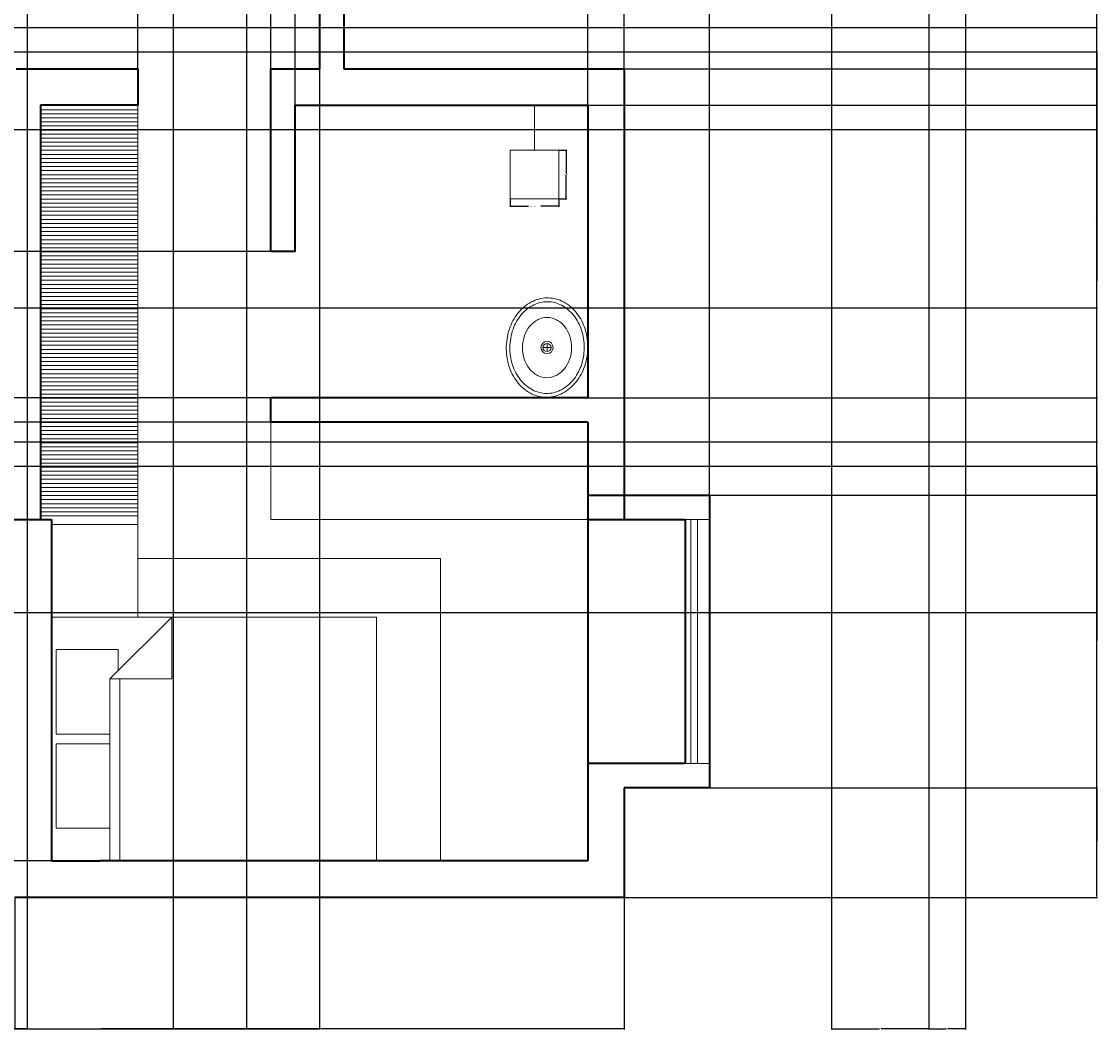
# Model space of a CAD drawing. Units: inches. Extents: x 1159 to 1869, y 2212 to 2738.
# Tile 4 of 5: x 1604 to 1869, y 2212 to 2460. Entities that reach past the tile are written whole.
import ezdxf

# ---------------------------------------------------------------- set-up
doc = ezdxf.new("R2010")
doc.units = ezdxf.units.IN
for name, color, linetype, lineweight in [('A-ANNO-DIMS', 2, 'Continuous', 18), ('A-FLOR', 9, 'Continuous', 13), ('A-FLOR-CASE', 30, 'Continuous', 18), ('A-FLOR-FIXT', 9, 'Continuous', 18), ('A-FLOR-PATT', 252, 'Continuous', 13), ('A-FURN', 8, 'Continuous', 18), ('A-GLAZ', 4, 'Continuous', 18), ('A-WALL', 7, 'Continuous', 35)]:
    doc.layers.add(name, color=color, linetype=linetype, lineweight=lineweight)
doc.styles.get("Standard").update_dxf_attribs({"font": 'arial.ttf'})
doc.dimstyles.get("Standard").update_dxf_attribs({"dimtxt": 0.18, "dimasz": 0.18, "dimexe": 0.18, "dimexo": 0.0625, "dimgap": 0.09, "dimtad": 0, "dimtih": 1, "dimtoh": 1, "dimdec": 4, "dimzin": 0, "dimdsep": 46, "dimtxsty": 'Standard', "dimcen": 0.09, "dimadec": 0, "dimazin": 0, "dimtfac": 1, "dimtdec": 4, "dimtofl": 0, "dimtmove": 0, "dimatfit": 3, "dimfxl": 1, "dimtolj": 1, "dimtzin": 0, "dimarcsym": 0})

# ---------------------------------------------------------------- blocks, each defined once
blk = doc.blocks.new('Bed - Queen')
for p, q in [((0, -80.00003), (0, 0)), ((0, 0), (59.99999, 0)), ((59.99999, 0), (59.99999, -80.00003)), ((7.99999, -1.2), (28.79998, -1.2)), ((7.99999, -14.4), (7.99999, -1.2)), ((28.79998, -1.2), (28.79998, -14.4)), ((31.19999, -1.2), (51.99999, -1.2)), ((31.19999, -14.4), (31.19999, -1.2)), ((51.99999, -1.2), (51.99999, -16.4)), ((0, -14.4), (44.8, -14.4)), ((59.99999, -29.6), (44.8, -14.4)), ((44.8, -14.4), (44.8, -29.6)), ((44.8, -16.8), (0, -16.8)), ((51.99999, -16.4), (46.79936, -16.4)), ((44.8, -29.6), (59.99999, -29.6)), ((59.99999, -80.00003), (0, -80.00003))]:
    blk.add_line(p, q)
blk = doc.blocks.new('Sink - Oval top')
for p, q in [((-1, 0), (1, 0)), ((0, 1), (0, -1))]:
    blk.add_line(p, q)
for points in [[(-12.23, 0.39, 0.117634), (-11.46, -3.36, 0.104469), (-8.88, -6.8, 0.090016), (-5.08, -9.07, 0.08192), (-0.32, -10.02, 0.08192), (4.49, -9.38, 0.090016), (8.42, -7.36, 0.104469), (11.22, -4.09, 0.117634), (12.23, -0.39, 0.117634), (11.46, 3.36, 0.104469), (8.88, 6.8, 0.090016), (5.08, 9.07, 0.08192), (0.32, 10.02, 0.08192), (-4.49, 9.38, 0.090016), (-8.42, 7.36, 0.104469), (-11.22, 4.09, 0.117634)], [(-11.29, 0.16, 0.118622), (-10.52, -3.25, 0.104678), (-8.07, -6.36, 0.089562), (-4.54, -8.37, 0.081185), (-0.13, -9.15, 0.081185), (4.3, -8.49, 0.089562), (7.89, -6.58, 0.104678), (10.42, -3.55, 0.118622), (11.29, -0.16, 0.118622), (10.52, 3.25, 0.104678), (8.07, 6.36, 0.089562), (4.54, 8.37, 0.081185), (0.13, 9.15, 0.081185), (-4.3, 8.49, 0.089562), (-7.89, 6.58, 0.104678), (-10.42, 3.55, 0.118622)], [(-7.42, 0.08, 0.118283), (-6.91, -2.17, 0.104607), (-5.29, -4.21, 0.089718), (-2.97, -5.53, 0.081436), (-0.07, -6.04, 0.081436), (2.84, -5.59, 0.089718), (5.2, -4.33, 0.104607), (6.86, -2.32, 0.118283), (7.42, -0.08, 0.118283), (6.91, 2.17, 0.104607), (5.29, 4.21, 0.089718), (2.97, 5.53, 0.081436), (0.07, 6.04, 0.081436), (-2.84, 5.59, 0.089718), (-5.2, 4.33, 0.104607), (-6.86, 2.32, 0.118283)]]:
    blk.add_lwpolyline(points, format="xyb", close=True)
for radius in [1.5, 1]:
    blk.add_circle((0, 0), radius)
blk = doc.blocks.new('SHOWER-HEAD-SQUARE-12IN')
for p, q in [((6, 12), (0, 12)), ((0, 12), (0, 0)), ((12, 12), (6, 12)), ((12, 0), (12, 12)), ((0, 0), (12, 0))]:
    blk.add_line(p, q)
blk = doc.blocks.new('*D12')
at = {"layer": 'A-ANNO-DIMS', "color": 0, "lineweight": -2, "transparency": 16777216}
for p, q in [((1724.31, 2415.97), (1724.31, 2414.05)), ((1736.31, 2415.97), (1736.31, 2414.05)), ((1724.49, 2414.23), (1728.8, 2414.23)), ((1736.13, 2414.23), (1731.82, 2414.23))]:
    blk.add_line(p, q, dxfattribs=at)
at = {"layer": 'A-ANNO-DIMS', "color": 0, "transparency": 16777216}
for points in [[(1724.49, 2414.26), (1724.49, 2414.2), (1724.31, 2414.23)], [(1736.13, 2414.26), (1736.13, 2414.2), (1736.31, 2414.23)]]:
    blk.add_solid(points, dxfattribs=at)
at = {"layer": 'Defpoints', "color": 0, "transparency": 16777216}
for p in [(1724.31, 2416.03), (1736.31, 2416.03), (1736.31, 2414.23)]:
    blk.add_point(p, dxfattribs=at)
at = {"layer": 'A-ANNO-DIMS', "color": 0, "transparency": 16777216, "insert": (1730.31, 2414.23), "char_height": 0.18, "attachment_point": 5}
blk.add_mtext('\\A1;SHOWER HEAD 12 TYP.', dxfattribs=at)
blk = doc.blocks.new('*D13')
at = {"layer": 'A-ANNO-DIMS', "color": 0, "lineweight": -2, "transparency": 16777216}
for p, q in [((1736.37, 2428.03), (1738.29, 2428.03)), ((1738.11, 2427.85), (1738.11, 2422.21)), ((1738.11, 2416.21), (1738.11, 2421.85)), ((1736.37, 2416.03), (1738.29, 2416.03))]:
    blk.add_line(p, q, dxfattribs=at)
at = {"layer": 'A-ANNO-DIMS', "color": 0, "transparency": 16777216}
for points in [[(1738.08, 2427.85), (1738.14, 2427.85), (1738.11, 2428.03)], [(1738.08, 2416.21), (1738.14, 2416.21), (1738.11, 2416.03)]]:
    blk.add_solid(points, dxfattribs=at)
at = {"layer": 'Defpoints', "color": 0, "transparency": 16777216}
for p in [(1736.31, 2428.03), (1738.11, 2428.03), (1736.31, 2416.03)]:
    blk.add_point(p, dxfattribs=at)
at = {"layer": 'A-ANNO-DIMS', "color": 0, "transparency": 16777216, "insert": (1738.11, 2422.03), "char_height": 0.18, "attachment_point": 5}
blk.add_mtext('\\A1;12 TYP.', dxfattribs=at)
blk = doc.blocks.new('*D21')
at = {"layer": 'A-ANNO-DIMS', "color": 0, "lineweight": -2, "transparency": 16777216}
for p, q in [((1836.46, 2705.63), (1868.92, 2705.63)), ((1868.74, 2705.45), (1868.74, 2475.03)), ((1868.74, 2244.26), (1868.74, 2474.67)), ((1752.46, 2244.08), (1868.92, 2244.08))]:
    blk.add_line(p, q, dxfattribs=at)
at = {"layer": 'A-ANNO-DIMS', "color": 0, "transparency": 16777216}
for points in [[(1868.71, 2705.45), (1868.77, 2705.45), (1868.74, 2705.63)], [(1868.71, 2244.26), (1868.77, 2244.26), (1868.74, 2244.08)]]:
    blk.add_solid(points, dxfattribs=at)
at = {"layer": 'Defpoints', "color": 0, "transparency": 16777216}
for p in [(1836.4, 2705.63), (1868.74, 2705.63), (1752.4, 2244.08)]:
    blk.add_point(p, dxfattribs=at)
at = {"layer": 'A-ANNO-DIMS', "color": 0, "transparency": 16777216, "insert": (1868.74, 2474.85), "char_height": 0.18, "attachment_point": 5}
blk.add_mtext('\\A1;461.55', dxfattribs=at)
blk = doc.blocks.new('*D28')
at = {"layer": 'A-ANNO-DIMS', "color": 0, "lineweight": -2, "transparency": 16777216}
for p, q in [((1602.4, 2244.01), (1602.4, 2211.56)), ((1752.4, 2244.01), (1752.4, 2211.56)), ((1602.58, 2211.74), (1677.12, 2211.74)), ((1752.22, 2211.74), (1677.68, 2211.74))]:
    blk.add_line(p, q, dxfattribs=at)
at = {"layer": 'A-ANNO-DIMS', "color": 0, "transparency": 16777216}
for points in [[(1602.58, 2211.77), (1602.58, 2211.71), (1602.4, 2211.74)], [(1752.22, 2211.77), (1752.22, 2211.71), (1752.4, 2211.74)]]:
    blk.add_solid(points, dxfattribs=at)
at = {"layer": 'Defpoints', "color": 0, "transparency": 16777216}
for p in [(1602.4, 2244.08), (1752.4, 2244.08), (1752.4, 2211.74)]:
    blk.add_point(p, dxfattribs=at)
at = {"layer": 'A-ANNO-DIMS', "color": 0, "transparency": 16777216, "insert": (1677.4, 2211.74), "char_height": 0.18, "attachment_point": 5}
blk.add_mtext('\\A1;150', dxfattribs=at)
blk = doc.blocks.new('*D31')
at = {"layer": 'A-ANNO-DIMS', "color": 0, "lineweight": -2, "transparency": 16777216}
for p, q in [((1698.46, 2519.63), (1868.92, 2519.63)), ((1868.74, 2519.45), (1868.74, 2484.03)), ((1868.74, 2448.26), (1868.74, 2483.67)), ((1683.46, 2448.08), (1868.92, 2448.08))]:
    blk.add_line(p, q, dxfattribs=at)
at = {"layer": 'A-ANNO-DIMS', "color": 0, "transparency": 16777216}
for points in [[(1868.71, 2519.45), (1868.77, 2519.45), (1868.74, 2519.63)], [(1868.71, 2448.26), (1868.77, 2448.26), (1868.74, 2448.08)]]:
    blk.add_solid(points, dxfattribs=at)
at = {"layer": 'Defpoints', "color": 0, "transparency": 16777216}
for p in [(1698.4, 2519.63), (1683.4, 2448.08), (1868.74, 2448.08)]:
    blk.add_point(p, dxfattribs=at)
at = {"layer": 'A-ANNO-DIMS', "color": 0, "transparency": 16777216, "insert": (1868.74, 2483.85), "char_height": 0.18, "attachment_point": 5}
blk.add_mtext('\\A1;71.55', dxfattribs=at)
blk = doc.blocks.new('*D33')
at = {"layer": 'A-ANNO-DIMS', "color": 0, "lineweight": -2, "transparency": 16777216}
for p, q in [((1773.46, 2271.08), (1868.92, 2271.08)), ((1868.74, 2270.9), (1868.74, 2257.76)), ((1868.74, 2244.26), (1868.74, 2257.4)), ((1752.46, 2244.08), (1868.92, 2244.08))]:
    blk.add_line(p, q, dxfattribs=at)
at = {"layer": 'A-ANNO-DIMS', "color": 0, "transparency": 16777216}
for points in [[(1868.71, 2270.9), (1868.77, 2270.9), (1868.74, 2271.08)], [(1868.71, 2244.26), (1868.77, 2244.26), (1868.74, 2244.08)]]:
    blk.add_solid(points, dxfattribs=at)
at = {"layer": 'Defpoints', "color": 0, "transparency": 16777216}
for p in [(1773.4, 2271.08), (1868.74, 2271.08), (1752.4, 2244.08)]:
    blk.add_point(p, dxfattribs=at)
at = {"layer": 'A-ANNO-DIMS', "color": 0, "transparency": 16777216, "insert": (1868.74, 2257.58), "char_height": 0.18, "attachment_point": 5}
blk.add_mtext('\\A1;27', dxfattribs=at)
blk = doc.blocks.new('*D34')
at = {"layer": 'A-ANNO-DIMS', "color": 0, "lineweight": -2, "transparency": 16777216}
for p, q in [((1773.46, 2343.08), (1868.92, 2343.08)), ((1868.74, 2342.9), (1868.74, 2307.26)), ((1868.74, 2271.26), (1868.74, 2306.9)), ((1773.46, 2271.08), (1868.92, 2271.08))]:
    blk.add_line(p, q, dxfattribs=at)
at = {"layer": 'A-ANNO-DIMS', "color": 0, "transparency": 16777216}
for points in [[(1868.71, 2342.9), (1868.77, 2342.9), (1868.74, 2343.08)], [(1868.71, 2271.26), (1868.77, 2271.26), (1868.74, 2271.08)]]:
    blk.add_solid(points, dxfattribs=at)
at = {"layer": 'Defpoints', "color": 0, "transparency": 16777216}
for p in [(1773.4, 2343.08), (1868.74, 2343.08), (1773.4, 2271.08)]:
    blk.add_point(p, dxfattribs=at)
at = {"layer": 'A-ANNO-DIMS', "color": 0, "transparency": 16777216, "insert": (1868.74, 2307.08), "char_height": 0.18, "attachment_point": 5}
blk.add_mtext('\\A1;72', dxfattribs=at)
blk = doc.blocks.new('*D35')
at = {"layer": 'A-ANNO-DIMS', "color": 0, "lineweight": -2, "transparency": 16777216}
for p, q in [((1752.46, 2448.08), (1868.92, 2448.08)), ((1868.74, 2447.9), (1868.74, 2395.76)), ((1868.74, 2343.26), (1868.74, 2395.39)), ((1773.46, 2343.08), (1868.92, 2343.08))]:
    blk.add_line(p, q, dxfattribs=at)
at = {"layer": 'A-ANNO-DIMS', "color": 0, "transparency": 16777216}
for points in [[(1868.71, 2447.9), (1868.77, 2447.9), (1868.74, 2448.08)], [(1868.71, 2343.26), (1868.77, 2343.26), (1868.74, 2343.08)]]:
    blk.add_solid(points, dxfattribs=at)
at = {"layer": 'Defpoints', "color": 0, "transparency": 16777216}
for p in [(1752.4, 2448.08), (1868.74, 2448.08), (1773.4, 2343.08)]:
    blk.add_point(p, dxfattribs=at)
at = {"layer": 'A-ANNO-DIMS', "color": 0, "transparency": 16777216, "insert": (1868.74, 2395.58), "char_height": 0.18, "attachment_point": 5}
blk.add_mtext('\\A1;105', dxfattribs=at)
blk = doc.blocks.new('*D36')
at = {"layer": 'A-ANNO-DIMS', "color": 0, "lineweight": -2, "transparency": 16777216}
for p, q in [((1752.4, 2337.14), (1752.4, 2738.15)), ((1752.58, 2737.97), (1762.7, 2737.97)), ((1773.22, 2737.97), (1763.1, 2737.97)), ((1773.4, 2343.14), (1773.4, 2738.15))]:
    blk.add_line(p, q, dxfattribs=at)
at = {"layer": 'A-ANNO-DIMS', "color": 0, "transparency": 16777216}
for points in [[(1752.58, 2738), (1752.58, 2737.94), (1752.4, 2737.97)], [(1773.22, 2738), (1773.22, 2737.94), (1773.4, 2737.97)]]:
    blk.add_solid(points, dxfattribs=at)
at = {"layer": 'Defpoints', "color": 0, "transparency": 16777216}
for p in [(1773.4, 2737.97), (1773.4, 2343.08), (1752.4, 2337.08)]:
    blk.add_point(p, dxfattribs=at)
at = {"layer": 'A-ANNO-DIMS', "color": 0, "transparency": 16777216, "insert": (1762.9, 2737.97), "char_height": 0.18, "attachment_point": 5}
blk.add_mtext('\\A1;21', dxfattribs=at)
blk = doc.blocks.new('*D39')
at = {"layer": 'A-ANNO-DIMS', "color": 0, "lineweight": -2, "transparency": 16777216}
for p, q in [((1605.4, 2696.57), (1605.4, 2211.56)), ((1677.4, 2696.57), (1677.4, 2211.56)), ((1605.58, 2211.74), (1641.18, 2211.74)), ((1677.22, 2211.74), (1641.62, 2211.74))]:
    blk.add_line(p, q, dxfattribs=at)
at = {"layer": 'A-ANNO-DIMS', "color": 0, "transparency": 16777216}
for points in [[(1605.58, 2211.77), (1605.58, 2211.71), (1605.4, 2211.74)], [(1677.22, 2211.77), (1677.22, 2211.71), (1677.4, 2211.74)]]:
    blk.add_solid(points, dxfattribs=at)
at = {"layer": 'Defpoints', "color": 0, "transparency": 16777216}
for p in [(1605.4, 2696.63), (1677.4, 2696.63), (1677.4, 2211.74)]:
    blk.add_point(p, dxfattribs=at)
at = {"layer": 'A-ANNO-DIMS', "color": 0, "transparency": 16777216, "insert": (1641.4, 2211.74), "char_height": 0.18, "attachment_point": 5}
blk.add_mtext('\\A1;72', dxfattribs=at)
blk = doc.blocks.new('*D42')
at = {"layer": 'A-ANNO-DIMS', "color": 0, "lineweight": -2, "transparency": 16777216}
for p, q in [((1200.46, 2452.21), (1868.92, 2452.21)), ((1868.74, 2452.03), (1868.74, 2404.39)), ((1868.74, 2356.39), (1868.74, 2404.02)), ((1200.46, 2356.21), (1868.92, 2356.21))]:
    blk.add_line(p, q, dxfattribs=at)
at = {"layer": 'A-ANNO-DIMS', "color": 0, "transparency": 16777216}
for points in [[(1868.71, 2452.03), (1868.77, 2452.03), (1868.74, 2452.21)], [(1868.71, 2356.39), (1868.77, 2356.39), (1868.74, 2356.21)]]:
    blk.add_solid(points, dxfattribs=at)
at = {"layer": 'Defpoints', "color": 0, "transparency": 16777216}
for p in [(1200.4, 2452.21), (1868.74, 2452.21), (1200.4, 2356.21)]:
    blk.add_point(p, dxfattribs=at)
at = {"layer": 'A-ANNO-DIMS', "color": 0, "transparency": 16777216, "insert": (1868.74, 2404.21), "char_height": 0.18, "attachment_point": 5}
blk.add_mtext('\\A1;96', dxfattribs=at)
blk = doc.blocks.new('*D43')
at = {"layer": 'A-ANNO-DIMS', "color": 0, "lineweight": -2, "transparency": 16777216}
for p, q in [((1671.4, 2439.14), (1671.4, 2738.15)), ((1671.58, 2737.97), (1707.18, 2737.97)), ((1743.22, 2737.97), (1707.62, 2737.97)), ((1743.4, 2439.14), (1743.4, 2738.15))]:
    blk.add_line(p, q, dxfattribs=at)
at = {"layer": 'A-ANNO-DIMS', "color": 0, "transparency": 16777216}
for points in [[(1671.58, 2738), (1671.58, 2737.94), (1671.4, 2737.97)], [(1743.22, 2738), (1743.22, 2737.94), (1743.4, 2737.97)]]:
    blk.add_solid(points, dxfattribs=at)
at = {"layer": 'Defpoints', "color": 0, "transparency": 16777216}
for p in [(1743.4, 2737.97), (1671.4, 2439.08), (1743.4, 2439.08)]:
    blk.add_point(p, dxfattribs=at)
at = {"layer": 'A-ANNO-DIMS', "color": 0, "transparency": 16777216, "insert": (1707.4, 2737.97), "char_height": 0.18, "attachment_point": 5}
blk.add_mtext('\\A1;72', dxfattribs=at)
blk = doc.blocks.new('*D44')
at = {"layer": 'A-ANNO-DIMS', "color": 0, "lineweight": -2, "transparency": 16777216}
for p, q in [((1671.46, 2439.08), (1868.92, 2439.08)), ((1868.74, 2438.9), (1868.74, 2403.26)), ((1868.74, 2367.26), (1868.74, 2402.9)), ((1671.46, 2367.08), (1868.92, 2367.08))]:
    blk.add_line(p, q, dxfattribs=at)
at = {"layer": 'A-ANNO-DIMS', "color": 0, "transparency": 16777216}
for points in [[(1868.71, 2438.9), (1868.77, 2438.9), (1868.74, 2439.08)], [(1868.71, 2367.26), (1868.77, 2367.26), (1868.74, 2367.08)]]:
    blk.add_solid(points, dxfattribs=at)
at = {"layer": 'Defpoints', "color": 0, "transparency": 16777216}
for p in [(1671.4, 2439.08), (1868.74, 2439.08), (1671.4, 2367.08)]:
    blk.add_point(p, dxfattribs=at)
at = {"layer": 'A-ANNO-DIMS', "color": 0, "transparency": 16777216, "insert": (1868.74, 2403.08), "char_height": 0.18, "attachment_point": 5}
blk.add_mtext('\\A1;72', dxfattribs=at)
blk = doc.blocks.new('*D53')
at = {"layer": 'A-ANNO-DIMS', "color": 0, "lineweight": -2, "transparency": 16777216}
for p, q in [((1425.46, 2504.63), (1868.92, 2504.63)), ((1868.74, 2504.45), (1868.74, 2481.6)), ((1868.74, 2458.39), (1868.74, 2481.24)), ((1428.81, 2458.21), (1868.92, 2458.21))]:
    blk.add_line(p, q, dxfattribs=at)
at = {"layer": 'A-ANNO-DIMS', "color": 0, "transparency": 16777216}
for points in [[(1868.71, 2504.45), (1868.77, 2504.45), (1868.74, 2504.63)], [(1868.71, 2458.39), (1868.77, 2458.39), (1868.74, 2458.21)]]:
    blk.add_solid(points, dxfattribs=at)
at = {"layer": 'Defpoints', "color": 0, "transparency": 16777216}
for p in [(1425.4, 2504.63), (1868.74, 2504.63), (1428.74, 2458.21)]:
    blk.add_point(p, dxfattribs=at)
at = {"layer": 'A-ANNO-DIMS', "color": 0, "transparency": 16777216, "insert": (1868.74, 2481.42), "char_height": 0.18, "attachment_point": 5}
blk.add_mtext('\\A1;46.42', dxfattribs=at)
blk = doc.blocks.new('*D58')
at = {"layer": 'A-ANNO-DIMS', "color": 0, "lineweight": -2, "transparency": 16777216}
for p, q in [((1538.03, 2433.09), (1868.92, 2433.09)), ((1868.74, 2432.91), (1868.74, 2411.32)), ((1868.74, 2389.36), (1868.74, 2410.95)), ((1538.03, 2389.18), (1868.92, 2389.18))]:
    blk.add_line(p, q, dxfattribs=at)
at = {"layer": 'A-ANNO-DIMS', "color": 0, "transparency": 16777216}
for points in [[(1868.71, 2432.91), (1868.77, 2432.91), (1868.74, 2433.09)], [(1868.71, 2389.36), (1868.77, 2389.36), (1868.74, 2389.18)]]:
    blk.add_solid(points, dxfattribs=at)
at = {"layer": 'Defpoints', "color": 0, "transparency": 16777216}
for p in [(1537.97, 2433.09), (1868.74, 2433.09), (1537.97, 2389.18)]:
    blk.add_point(p, dxfattribs=at)
at = {"layer": 'A-ANNO-DIMS', "color": 0, "transparency": 16777216, "insert": (1868.74, 2411.14), "char_height": 0.18, "attachment_point": 5}
blk.add_mtext('\\A1;43.92', dxfattribs=at)
blk = doc.blocks.new('*D60')
at = {"layer": 'A-ANNO-DIMS', "color": 0, "lineweight": -2, "transparency": 16777216}
for p, q in [((1659.4, 2552.57), (1659.4, 2211.56)), ((1605.4, 2549.57), (1605.4, 2211.56)), ((1605.58, 2211.74), (1632.18, 2211.74)), ((1659.22, 2211.74), (1632.62, 2211.74))]:
    blk.add_line(p, q, dxfattribs=at)
at = {"layer": 'A-ANNO-DIMS', "color": 0, "transparency": 16777216}
for points in [[(1605.58, 2211.77), (1605.58, 2211.71), (1605.4, 2211.74)], [(1659.22, 2211.77), (1659.22, 2211.71), (1659.4, 2211.74)]]:
    blk.add_solid(points, dxfattribs=at)
at = {"layer": 'Defpoints', "color": 0, "transparency": 16777216}
for p in [(1659.4, 2552.63), (1605.4, 2549.63), (1605.4, 2211.74)]:
    blk.add_point(p, dxfattribs=at)
at = {"layer": 'A-ANNO-DIMS', "color": 0, "transparency": 16777216, "insert": (1632.4, 2211.74), "char_height": 0.18, "attachment_point": 5}
blk.add_mtext('\\A1;54', dxfattribs=at)
blk = doc.blocks.new('*D61')
at = {"layer": 'A-ANNO-DIMS', "color": 0, "lineweight": -2, "transparency": 16777216}
for p, q in [((1632.68, 2448.14), (1632.68, 2738.15)), ((1632.86, 2737.97), (1648.65, 2737.97)), ((1665.22, 2737.97), (1649.43, 2737.97)), ((1665.4, 2448.14), (1665.4, 2738.15))]:
    blk.add_line(p, q, dxfattribs=at)
at = {"layer": 'A-ANNO-DIMS', "color": 0, "transparency": 16777216}
for points in [[(1632.86, 2738), (1632.86, 2737.94), (1632.68, 2737.97)], [(1665.22, 2738), (1665.22, 2737.94), (1665.4, 2737.97)]]:
    blk.add_solid(points, dxfattribs=at)
at = {"layer": 'Defpoints', "color": 0, "transparency": 16777216}
for p in [(1665.4, 2737.97), (1632.68, 2448.08), (1665.4, 2448.08)]:
    blk.add_point(p, dxfattribs=at)
at = {"layer": 'A-ANNO-DIMS', "color": 0, "transparency": 16777216, "insert": (1649.04, 2737.97), "char_height": 0.18, "attachment_point": 5}
blk.add_mtext('\\A1;32.72', dxfattribs=at)
blk = doc.blocks.new('*D65')
at = {"layer": 'A-ANNO-DIMS', "color": 0, "lineweight": -2, "transparency": 16777216}
for p, q in [((1542.76, 2504.57), (1542.76, 2211.56)), ((1605.4, 2504.57), (1605.4, 2211.56)), ((1542.94, 2211.74), (1573.69, 2211.74)), ((1605.22, 2211.74), (1574.48, 2211.74))]:
    blk.add_line(p, q, dxfattribs=at)
at = {"layer": 'A-ANNO-DIMS', "color": 0, "transparency": 16777216}
for points in [[(1542.94, 2211.77), (1542.94, 2211.71), (1542.76, 2211.74)], [(1605.22, 2211.77), (1605.22, 2211.71), (1605.4, 2211.74)]]:
    blk.add_solid(points, dxfattribs=at)
at = {"layer": 'Defpoints', "color": 0, "transparency": 16777216}
for p in [(1542.76, 2504.63), (1605.4, 2504.63), (1605.4, 2211.74)]:
    blk.add_point(p, dxfattribs=at)
at = {"layer": 'A-ANNO-DIMS', "color": 0, "transparency": 16777216, "insert": (1574.08, 2211.74), "char_height": 0.18, "attachment_point": 5}
blk.add_mtext('\\A1;62.64', dxfattribs=at)
blk = doc.blocks.new('*D66')
at = {"layer": 'A-ANNO-DIMS', "color": 0, "lineweight": -2, "transparency": 16777216}
for p, q in [((1605.4, 2696.57), (1605.4, 2211.56)), ((1641.4, 2600.57), (1641.4, 2211.56)), ((1605.58, 2211.74), (1623.18, 2211.74)), ((1641.22, 2211.74), (1623.62, 2211.74))]:
    blk.add_line(p, q, dxfattribs=at)
at = {"layer": 'A-ANNO-DIMS', "color": 0, "transparency": 16777216}
for points in [[(1605.58, 2211.77), (1605.58, 2211.71), (1605.4, 2211.74)], [(1641.22, 2211.77), (1641.22, 2211.71), (1641.4, 2211.74)]]:
    blk.add_solid(points, dxfattribs=at)
at = {"layer": 'Defpoints', "color": 0, "transparency": 16777216}
for p in [(1605.4, 2696.63), (1641.4, 2600.63), (1605.4, 2211.74)]:
    blk.add_point(p, dxfattribs=at)
at = {"layer": 'A-ANNO-DIMS', "color": 0, "transparency": 16777216, "insert": (1623.4, 2211.74), "char_height": 0.18, "attachment_point": 5}
blk.add_mtext('\\A1;36', dxfattribs=at)
blk = doc.blocks.new('*D67')
at = {"layer": 'A-ANNO-DIMS', "color": 0, "lineweight": -2, "transparency": 16777216}
for p, q in [((1665.34, 2403.08), (1158.88, 2403.08)), ((1159.06, 2402.9), (1159.06, 2385.26)), ((1159.06, 2367.26), (1159.06, 2384.89)), ((1665.34, 2367.08), (1158.88, 2367.08))]:
    blk.add_line(p, q, dxfattribs=at)
at = {"layer": 'A-ANNO-DIMS', "color": 0, "transparency": 16777216}
for points in [[(1159.03, 2402.9), (1159.09, 2402.9), (1159.06, 2403.08)], [(1159.03, 2367.26), (1159.09, 2367.26), (1159.06, 2367.08)]]:
    blk.add_solid(points, dxfattribs=at)
at = {"layer": 'Defpoints', "color": 0, "transparency": 16777216}
for p in [(1159.06, 2403.08), (1665.4, 2403.08), (1665.4, 2367.08)]:
    blk.add_point(p, dxfattribs=at)
at = {"layer": 'A-ANNO-DIMS', "color": 0, "transparency": 16777216, "insert": (1159.06, 2385.08), "char_height": 0.18, "attachment_point": 5}
blk.add_mtext('\\A1;36', dxfattribs=at)
blk = doc.blocks.new('*D68')
at = {"layer": 'A-ANNO-DIMS', "color": 0, "lineweight": -2, "transparency": 16777216}
for p, q in [((1803.4, 2552.57), (1803.4, 2211.56)), ((1827.4, 2552.57), (1827.4, 2211.56)), ((1803.58, 2211.74), (1815.18, 2211.74)), ((1827.22, 2211.74), (1815.62, 2211.74))]:
    blk.add_line(p, q, dxfattribs=at)
at = {"layer": 'A-ANNO-DIMS', "color": 0, "transparency": 16777216}
for points in [[(1803.58, 2211.77), (1803.58, 2211.71), (1803.4, 2211.74)], [(1827.22, 2211.77), (1827.22, 2211.71), (1827.4, 2211.74)]]:
    blk.add_solid(points, dxfattribs=at)
at = {"layer": 'Defpoints', "color": 0, "transparency": 16777216}
for p in [(1803.4, 2552.63), (1827.4, 2552.63), (1827.4, 2211.74)]:
    blk.add_point(p, dxfattribs=at)
at = {"layer": 'A-ANNO-DIMS', "color": 0, "transparency": 16777216, "insert": (1815.4, 2211.74), "char_height": 0.18, "attachment_point": 5}
blk.add_mtext('\\A1;24', dxfattribs=at)
blk = doc.blocks.new('*D70')
at = {"layer": 'A-ANNO-DIMS', "color": 0, "lineweight": -2, "transparency": 16777216}
for p, q in [((1827.4, 2528.57), (1827.4, 2211.56)), ((1836.4, 2519.57), (1836.4, 2211.56)), ((1827.58, 2211.74), (1831.75, 2211.74)), ((1836.22, 2211.74), (1832.05, 2211.74))]:
    blk.add_line(p, q, dxfattribs=at)
at = {"layer": 'A-ANNO-DIMS', "color": 0, "transparency": 16777216}
for points in [[(1827.58, 2211.77), (1827.58, 2211.71), (1827.4, 2211.74)], [(1836.22, 2211.77), (1836.22, 2211.71), (1836.4, 2211.74)]]:
    blk.add_solid(points, dxfattribs=at)
at = {"layer": 'Defpoints', "color": 0, "transparency": 16777216}
for p in [(1827.4, 2528.63), (1836.4, 2519.63), (1836.4, 2211.74)]:
    blk.add_point(p, dxfattribs=at)
at = {"layer": 'A-ANNO-DIMS', "color": 0, "transparency": 16777216, "insert": (1831.9, 2211.74), "char_height": 0.18, "attachment_point": 5}
blk.add_mtext('\\A1;9', dxfattribs=at)
blk = doc.blocks.new('*D71')
at = {"layer": 'A-ANNO-DIMS', "color": 0, "lineweight": -2, "transparency": 16777216}
for p, q in [((1677.4, 2448.14), (1677.4, 2738.15)), ((1677.58, 2737.97), (1680.25, 2737.97)), ((1683.22, 2737.97), (1680.55, 2737.97)), ((1683.4, 2448.14), (1683.4, 2738.15))]:
    blk.add_line(p, q, dxfattribs=at)
at = {"layer": 'A-ANNO-DIMS', "color": 0, "transparency": 16777216}
for points in [[(1677.58, 2738), (1677.58, 2737.94), (1677.4, 2737.97)], [(1683.22, 2738), (1683.22, 2737.94), (1683.4, 2737.97)]]:
    blk.add_solid(points, dxfattribs=at)
at = {"layer": 'Defpoints', "color": 0, "transparency": 16777216}
for p in [(1683.4, 2737.97), (1677.4, 2448.08), (1683.4, 2448.08)]:
    blk.add_point(p, dxfattribs=at)
at = {"layer": 'A-ANNO-DIMS', "color": 0, "transparency": 16777216, "insert": (1680.4, 2737.97), "char_height": 0.18, "attachment_point": 5}
blk.add_mtext('\\A1;6', dxfattribs=at)
blk = doc.blocks.new('*D74')
at = {"layer": 'A-ANNO-DIMS', "color": 0, "lineweight": -2, "transparency": 16777216}
for p, q in [((1743.34, 2361.08), (1158.88, 2361.08)), ((1159.06, 2360.9), (1159.06, 2307.26)), ((1159.06, 2253.26), (1159.06, 2306.89)), ((1743.34, 2253.08), (1158.88, 2253.08))]:
    blk.add_line(p, q, dxfattribs=at)
at = {"layer": 'A-ANNO-DIMS', "color": 0, "transparency": 16777216}
for points in [[(1159.03, 2360.9), (1159.09, 2360.9), (1159.06, 2361.08)], [(1159.03, 2253.26), (1159.09, 2253.26), (1159.06, 2253.08)]]:
    blk.add_solid(points, dxfattribs=at)
at = {"layer": 'Defpoints', "color": 0, "transparency": 16777216}
for p in [(1159.06, 2361.08), (1743.4, 2361.08), (1743.4, 2253.08)]:
    blk.add_point(p, dxfattribs=at)
at = {"layer": 'A-ANNO-DIMS', "color": 0, "transparency": 16777216, "insert": (1159.06, 2307.08), "char_height": 0.18, "attachment_point": 5}
blk.add_mtext('\\A1;108', dxfattribs=at)
blk = doc.blocks.new('*D75')
at = {"layer": 'A-ANNO-DIMS', "color": 0, "lineweight": -2, "transparency": 16777216}
for p, q in [((1227.43, 2350.21), (1868.92, 2350.21)), ((1868.74, 2350.03), (1868.74, 2332.39)), ((1868.74, 2314.39), (1868.74, 2332.02)), ((1227.43, 2314.21), (1868.92, 2314.21))]:
    blk.add_line(p, q, dxfattribs=at)
at = {"layer": 'A-ANNO-DIMS', "color": 0, "transparency": 16777216}
for points in [[(1868.71, 2350.03), (1868.77, 2350.03), (1868.74, 2350.21)], [(1868.71, 2314.39), (1868.77, 2314.39), (1868.74, 2314.21)]]:
    blk.add_solid(points, dxfattribs=at)
at = {"layer": 'Defpoints', "color": 0, "transparency": 16777216}
for p in [(1227.37, 2350.21), (1868.74, 2350.21), (1227.37, 2314.21)]:
    blk.add_point(p, dxfattribs=at)
at = {"layer": 'A-ANNO-DIMS', "color": 0, "transparency": 16777216, "insert": (1868.74, 2332.21), "char_height": 0.18, "attachment_point": 5}
blk.add_mtext('\\A1;36', dxfattribs=at)

msp = doc.modelspace()

# ---------------------------------------------------------------- hatches: boundary and pattern name
at = {"layer": 'A-FLOR-PATT'}
h = msp.add_hatch(dxfattribs=at)
h.set_pattern_fill('ANSI31', color=256, scale=0.3149606, angle=-45, style=0)
h.paths.add_polyline_path([(1608.6806, 2337.0757), (1632.6806, 2337.0757), (1632.6806, 2439.0757), (1608.6806, 2439.0757)])

# ---------------------------------------------------------------- linework, layer by layer
at = {"layer": 'A-FLOR'}
for p, q in [((1632.6806, 2327.4793), (1707.2045, 2327.4793)), ((1707.2045, 2327.4793), (1707.2045, 2253.0757))]:
    msp.add_line(p, q, dxfattribs=at)
at = {"layer": 'A-FLOR-CASE'}
for p, q in [((1632.6806, 2439.0757), (1632.6806, 2313.0757)), ((1665.4011, 2361.0757), (1665.4011, 2337.0757)), ((1611.4011, 2335.8952), (1632.6806, 2335.8952)), ((1743.4011, 2337.0757), (1665.4011, 2337.0757))]:
    msp.add_line(p, q, dxfattribs=at)
at = {"layer": 'A-FLOR-FIXT'}
msp.add_line((1730.3083, 2439.0757), (1730.3083, 2428.0287), dxfattribs=at)
at = {"layer": 'A-GLAZ'}
for p, q in [((1767.4011, 2337.0757), (1773.4011, 2337.0757)), ((1768.7428, 2277.0757), (1768.7428, 2337.0757)), ((1770.4011, 2337.0757), (1770.4011, 2277.0757)), ((1767.4011, 2277.0757), (1773.4011, 2277.0757))]:
    msp.add_line(p, q, dxfattribs=at)
at = {"layer": 'A-WALL'}
for p, q in [((1677.4011, 2543.6279), (1677.4011, 2448.0757)), ((1683.4011, 2543.6279), (1683.4011, 2448.0757)), ((1602.6806, 2448.0757), (1632.6806, 2448.0757)), ((1632.6806, 2448.0757), (1632.6806, 2439.0757)), ((1665.4011, 2439.0757), (1665.4011, 2448.0757)), ((1665.4011, 2448.0757), (1677.4011, 2448.0757)), ((1683.4011, 2448.0757), (1752.4011, 2448.0757)), ((1752.4011, 2448.0757), (1752.4011, 2337.0757)), ((1632.6806, 2439.0757), (1608.6806, 2439.0757)), ((1608.6806, 2439.0757), (1608.6806, 2337.0757)), ((1665.4011, 2403.0757), (1665.4011, 2439.0757)), ((1671.4011, 2403.0757), (1671.4011, 2439.0757)), ((1671.4011, 2439.0757), (1677.4011, 2439.0757)), ((1677.4011, 2439.0757), (1683.4011, 2439.0757)), ((1683.4011, 2439.0757), (1743.4011, 2439.0757)), ((1743.4011, 2439.0757), (1743.4011, 2367.0757)), ((1671.4011, 2403.0757), (1665.4011, 2403.0757)), ((1665.4011, 2361.0757), (1665.4011, 2367.0757)), ((1671.4011, 2367.0757), (1665.4011, 2367.0757)), ((1743.4011, 2367.0757), (1671.4011, 2367.0757)), ((1743.4011, 2361.0757), (1665.4011, 2361.0757)), ((1743.4011, 2361.0757), (1743.4011, 2337.0757)), ((1743.4011, 2343.0757), (1773.4011, 2343.0757)), ((1773.4011, 2343.0757), (1773.4011, 2271.0757)), ((1494.4011, 2337.0757), (1611.4011, 2337.0757)), ((1611.4011, 2337.0757), (1611.4011, 2253.0757)), ((1743.4011, 2337.0757), (1767.4011, 2337.0757)), ((1743.4011, 2337.0757), (1743.4011, 2277.0757)), ((1767.4011, 2337.0757), (1767.4011, 2277.0757)), ((1767.4011, 2277.0757), (1743.4011, 2277.0757)), ((1743.4011, 2277.0757), (1743.4011, 2253.0757)), ((1752.4011, 2271.0757), (1752.4011, 2244.0757)), ((1773.4011, 2271.0757), (1752.4011, 2271.0757)), ((1611.4011, 2253.0757), (1623.4011, 2253.0757)), ((1743.4011, 2253.0757), (1623.4011, 2253.0757)), ((1614.4011, 2244.0757), (1602.4011, 2244.0757)), ((1752.4011, 2244.0757), (1614.4011, 2244.0757))]:
    msp.add_line(p, q, dxfattribs=at)

# ---------------------------------------------------------------- block references
at = {"layer": 'A-FLOR-FIXT'}
msp.add_blockref('SHOWER-HEAD-SQUARE-12IN', (1724.308, 2416.029), dxfattribs=at)
at = {"layer": 'A-FLOR-FIXT', "rotation": 90}
msp.add_blockref('Sink - Oval top', (1733.3853, 2379.438), dxfattribs=at)
at = {"layer": 'A-FURN', "rotation": 90}
msp.add_blockref('Bed - Queen', (1611.4011, 2253.0757), dxfattribs=at)

# ---------------------------------------------------------------- dimensions: what is measured, and where the dimension line sits
at = {"layer": 'A-ANNO-DIMS'}
for base, p1, p2, override, picture, middle in [((1665.4011, 2737.9679), (1632.6806, 2448.0757), (1665.4011, 2448.0757), {"dimdec": 2, "dimlfac": 1, "dimrnd": 0, "dimzin": 0, "dimdsep": 46, "dimlunit": 2}, '*D61', (1649.0408, 2737.9679)), ((1743.4011, 2737.9679), (1671.4011, 2439.0757), (1743.4011, 2439.0757), {"dimdec": 0, "dimlfac": 1, "dimrnd": 0, "dimzin": 0, "dimdsep": 46, "dimlunit": 2}, '*D43', (1707.4011, 2737.9679)), ((1683.4011, 2737.9679), (1677.4011, 2448.0757), (1683.4011, 2448.0757), {"dimdec": 0, "dimlfac": 1, "dimrnd": 0, "dimzin": 0, "dimdsep": 46, "dimlunit": 2}, '*D71', (1680.4011, 2737.9679)), ((1773.4011, 2737.9679), (1752.4011, 2337.0757), (1773.4011, 2343.0757), {"dimdec": 0, "dimlfac": 1, "dimrnd": 0, "dimzin": 0, "dimdsep": 46, "dimlunit": 2}, '*D36', (1762.9011, 2737.9679)), ((1677.4011, 2211.7357), (1605.4011, 2696.6279), (1677.4011, 2696.6279), {"dimdec": 0, "dimlfac": 1, "dimrnd": 0, "dimzin": 0, "dimdsep": 46, "dimlunit": 2}, '*D39', (1641.4011, 2211.7357)), ((1605.4011, 2211.7357), (1641.4011, 2600.6279), (1605.4011, 2696.6279), {"dimdec": 0, "dimlfac": 1, "dimrnd": 0, "dimzin": 0, "dimdsep": 46, "dimlunit": 2}, '*D66', (1623.4011, 2211.7357)), ((1605.4011, 2211.7357), (1659.4011, 2552.6279), (1605.4011, 2549.6279), {"dimdec": 0, "dimlfac": 1, "dimrnd": 0, "dimzin": 0, "dimdsep": 46, "dimlunit": 2}, '*D60', (1632.4011, 2211.7357)), ((1827.4011, 2211.7357), (1803.4011, 2552.6279), (1827.4011, 2552.6279), {"dimdec": 0, "dimlfac": 1, "dimrnd": 0, "dimzin": 0, "dimdsep": 46, "dimlunit": 2}, '*D68', (1815.4011, 2211.7357)), ((1836.4011, 2211.7357), (1827.4011, 2528.6279), (1836.4011, 2519.6279), {"dimdec": 0, "dimlfac": 1, "dimrnd": 0, "dimzin": 0, "dimdsep": 46, "dimlunit": 2}, '*D70', (1831.9011, 2211.7357)), ((1605.4011, 2211.7357), (1542.764, 2504.6279), (1605.4011, 2504.6279), {"dimdec": 2, "dimlfac": 1, "dimrnd": 0, "dimzin": 0, "dimdsep": 46, "dimlunit": 2}, '*D65', (1574.0826, 2211.7357)), ((1752.4011, 2211.7357), (1602.4011, 2244.0757), (1752.4011, 2244.0757), {"dimdec": 0, "dimlfac": 1, "dimrnd": 0, "dimzin": 0, "dimdsep": 46, "dimlunit": 2}, '*D28', (1677.4011, 2211.7357))]:
    dim = msp.add_linear_dim(base=base, p1=p1, p2=p2, dimstyle='Standard', override=override, dxfattribs=at)
    dim.commit()
    dim.dimension.update_dxf_attribs({"geometry": picture, "text_midpoint": middle})
for base, p1, p2, override, picture, middle in [((1868.7411, 2705.6279), (1752.4011, 2244.0757), (1836.4011, 2705.6279), {"dimdec": 2, "dimlfac": 1, "dimrnd": 0, "dimzin": 0, "dimdsep": 46, "dimlunit": 2}, '*D21', (1868.7411, 2474.8518)), ((1868.7411, 2448.0757), (1698.4011, 2519.6279), (1683.4011, 2448.0757), {"dimdec": 2, "dimlfac": 1, "dimrnd": 0, "dimzin": 0, "dimdsep": 46, "dimlunit": 2}, '*D31', (1868.7411, 2483.8518)), ((1868.7411, 2504.6279), (1428.7443, 2458.2064), (1425.4011, 2504.6279), {"dimdec": 2, "dimlfac": 1, "dimrnd": 0, "dimzin": 0, "dimdsep": 46, "dimlunit": 2}, '*D53', (1868.7411, 2481.4172)), ((1868.7411, 2452.2064), (1200.4011, 2356.2064), (1200.4011, 2452.2064), {"dimdec": 0, "dimlfac": 1, "dimrnd": 0, "dimzin": 0, "dimdsep": 46, "dimlunit": 2}, '*D42', (1868.7411, 2404.2064)), ((1868.7411, 2448.0757), (1773.4011, 2343.0757), (1752.4011, 2448.0757), {"dimdec": 0, "dimlfac": 1, "dimrnd": 0, "dimzin": 0, "dimdsep": 46, "dimlunit": 2}, '*D35', (1868.7411, 2395.5757)), ((1868.7411, 2439.0757), (1671.4011, 2367.0757), (1671.4011, 2439.0757), {"dimdec": 0, "dimlfac": 1, "dimrnd": 0, "dimzin": 0, "dimdsep": 46, "dimlunit": 2}, '*D44', (1868.7411, 2403.0757)), ((1868.7411, 2433.0936), (1537.9722, 2389.1774), (1537.9722, 2433.0936), {"dimdec": 2, "dimlfac": 1, "dimrnd": 0, "dimzin": 0, "dimdsep": 46, "dimlunit": 2}, '*D58', (1868.7411, 2411.1355)), ((1159.0611, 2403.0757), (1665.4011, 2367.0757), (1665.4011, 2403.0757), {"dimdec": 0, "dimlfac": 1, "dimrnd": 0, "dimzin": 0, "dimdsep": 46, "dimlunit": 2}, '*D67', (1159.0611, 2385.0757)), ((1159.0611, 2361.0757), (1743.4011, 2253.0757), (1743.4011, 2361.0757), {"dimdec": 0, "dimlfac": 1, "dimrnd": 0, "dimzin": 0, "dimdsep": 46, "dimlunit": 2}, '*D74', (1159.0611, 2307.0757)), ((1868.7411, 2350.2064), (1227.3685, 2314.2064), (1227.3685, 2350.2064), {"dimdec": 0, "dimlfac": 1, "dimrnd": 0, "dimzin": 0, "dimdsep": 46, "dimlunit": 2}, '*D75', (1868.7411, 2332.2064)), ((1868.7411, 2343.0757), (1773.4011, 2271.0757), (1773.4011, 2343.0757), {"dimdec": 0, "dimlfac": 1, "dimrnd": 0, "dimzin": 0, "dimdsep": 46, "dimlunit": 2}, '*D34', (1868.7411, 2307.0757)), ((1868.7411, 2271.0757), (1752.4011, 2244.0757), (1773.4011, 2271.0757), {"dimdec": 0, "dimlfac": 1, "dimrnd": 0, "dimzin": 0, "dimdsep": 46, "dimlunit": 2}, '*D33', (1868.7411, 2257.5757))]:
    dim = msp.add_linear_dim(base=base, p1=p1, p2=p2, angle=90, dimstyle='Standard', override=override, dxfattribs=at)
    dim.commit()
    dim.dimension.update_dxf_attribs({"geometry": picture, "text_midpoint": middle})
dim = msp.add_linear_dim(base=(1738.1083, 2428.0287), p1=(1736.3083, 2416.0287), p2=(1736.3083, 2428.0287), angle=90, text='<> TYP.', dimstyle='Standard', override={"dimdec": 0, "dimlfac": 1, "dimrnd": 0, "dimzin": 0, "dimdsep": 46, "dimlunit": 2}, dxfattribs=at)
dim.commit()
dim.dimension.update_dxf_attribs({"geometry": '*D13', "text_midpoint": (1738.1083, 2422.0287)})
dim = msp.add_linear_dim(base=(1736.3083, 2414.2287), p1=(1724.3083, 2416.0287), p2=(1736.3083, 2416.0287), text='SHOWER HEAD <> TYP.', dimstyle='Standard', override={"dimdec": 0, "dimlfac": 1, "dimrnd": 0, "dimzin": 0, "dimdsep": 46, "dimlunit": 2}, dxfattribs=at)
dim.commit()
dim.dimension.update_dxf_attribs({"geometry": '*D12', "text_midpoint": (1730.3083, 2414.2287)})

doc.saveas('drawing.dxf')
